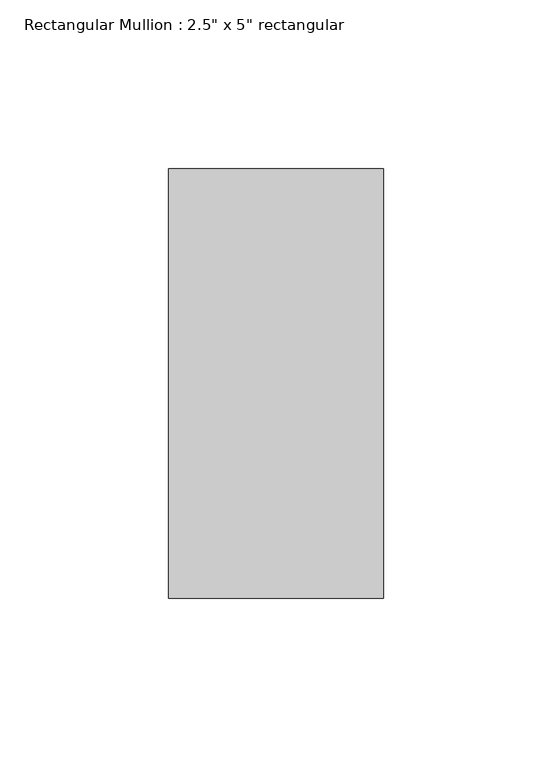
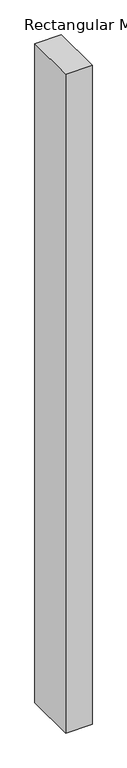
"""IFC4 building model written with IfcOpenShell, lengths in millimetres: member geometry."""

from ifc_helpers import new_model, si_unit, frame, origin, place, context, project, spatial, polyline, outline, extrude, source, transform, mapped, element, save


def member_f9446df5(model_context):
    return source(origin(), model_context, "Body", "SweptSolid", [
        extrude(outline(polyline([(31.75, 63.5), (31.75, -63.5), (-31.75, -63.5), (-31.75, 63.5), (31.75, 63.5)])), frame((0.0, 0.0, -1667.45282), z_axis=(0.0, 0.0, 1.0), x_axis=(1.0, 0.0, 0.0)), (0.0, 0.0, 1.0), 1667.45282),
    ])


if __name__ == "__main__":
    model = new_model("IFC4")
    model_context = context("Model", 3, world=origin())
    ifc_project = project(units=[si_unit("LENGTHUNIT", "METRE", prefix="MILLI")], contexts=[model_context])
    site = spatial("IfcSite", under=ifc_project)
    building = spatial("IfcBuilding", under=site)
    placement = place(None, origin())
    member_shape = member_f9446df5(model_context)
    element("IfcMember", 1, ObjectType="Rectangular Mullion : 2.5\" x 5\" rectangular", at=placement, inside=building, context=model_context, shape_type="MappedRepresentation", body=[
        mapped(member_shape, transform((0.0, 0.0, 0.0), x_axis=(1.0, 0.0, 0.0), y_axis=(0.0, 1.0, 0.0), z_axis=(0.0, 0.0, 1.0))),
    ])
    save(model, "model.ifc")

# Revit data of these elements
# Type "Rectangular Mullion : 2.5\" x 5\" rectangular"
#   built-in parameter 1007304 = 0.416667 (stored number, unit not read)
#   built-in parameter 1007301 = 0.104167 (stored number, unit not read)
#   built-in parameter 1007300 = 0.104167 (stored number, unit not read)
# Element 1 (IfcMember, "Rectangular Mullion : 2.5\" x 5\" rectangular")
#   Materials on its faces: "Aluminum"
# Materials
#   "Aluminum": class "Metal", colour RGB 247 247 247, transparency 0, Description = "Aluminum 6061", Cost = 0
